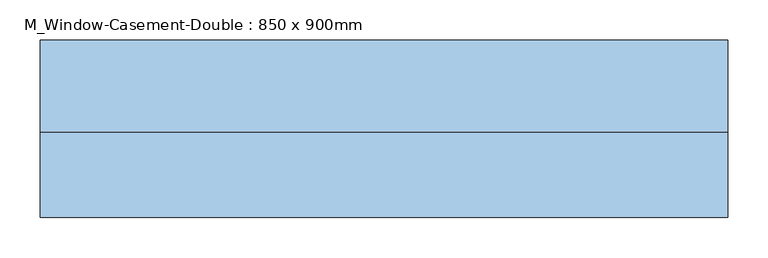
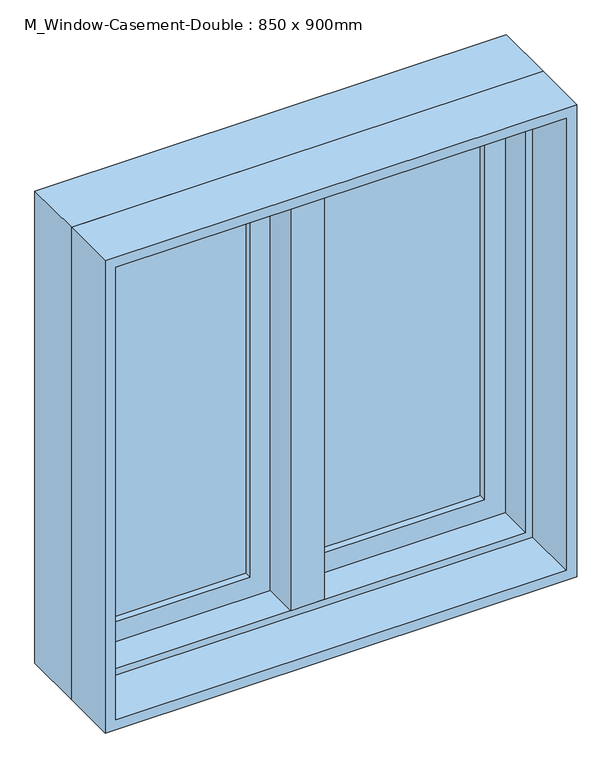
"""IFC4 building model written with IfcOpenShell, lengths in millimetres: window geometry, M_Window-Casement-Double : 850 x 900mm."""

from ifc_helpers import new_model, si_unit, frame, origin, place, context, project, spatial, polyline, outline, extrude, faceted_brep, source, transform, mapped, element, save


def m_window_casement_double_850_x_900mm_0f766704(model_context):
    return source(origin(), model_context, "Body", "SolidModel", [
        faceted_brep([(9.525, 119.05, 1787.3), (-9.525, 119.05, 1787.3), (-9.525, 68.25, 1787.3), (9.525, 68.25, 1787.3), (9.525, 119.05, 912.7), (9.525, 68.25, 912.7), (-9.525, 68.25, 912.7), (-9.525, 119.05, 912.7), (-9.525, 68.25, 931.75), (-9.525, 68.25, 1768.25), (-30.1625, 68.25, 931.75), (-30.1625, 68.25, 1768.25), (-30.1625, 4.75, 931.75), (-30.1625, 4.75, 1768.25), (30.1625, 4.75, 931.75), (30.1625, 4.75, 1768.25), (30.1625, 68.25, 931.75), (30.1625, 68.25, 1768.25), (9.525, 68.25, 931.75), (9.525, 68.25, 1768.25)], [[[0, 1, 2, 3]], [[4, 5, 6, 7]], [[1, 0, 4, 7]], [[2, 1, 7, 6, 8, 9]], [[9, 8, 10, 11]], [[11, 10, 12, 13]], [[13, 12, 14, 15]], [[15, 14, 16, 17]], [[17, 16, 18, 19]], [[0, 3, 19, 18, 5, 4]], [[18, 8, 6, 5]], [[9, 19, 3, 2]], [[8, 18, 16, 14, 12, 10]], [[19, 9, 11, 13, 15, 17]]]),
        extrude(outline(polyline([(-66.675, 100.0), (-66.675, 93.65), (-355.15, 93.65), (-355.15, 100.0), (-66.675, 100.0)])), frame((0.0, 0.0, 969.85), z_axis=(0.0, 0.0, 1.0), x_axis=(1.0, 0.0, 0.0)), (0.0, 0.0, 1.0), 760.3),
        extrude(outline(polyline([(-355.15, 80.95), (-355.15, 87.3), (-66.675, 87.3), (-66.675, 80.95), (-355.15, 80.95)])), frame((0.0, 0.0, 969.85), z_axis=(0.0, 0.0, 1.0), x_axis=(1.0, 0.0, 0.0)), (0.0, 0.0, 1.0), 760.3),
        extrude(outline(polyline([(355.15, 100.0), (355.15, 93.65), (66.675, 93.65), (66.675, 100.0), (355.15, 100.0)])), frame((0.0, 0.0, 969.85), z_axis=(0.0, 0.0, 1.0), x_axis=(1.0, 0.0, 0.0)), (0.0, 0.0, 1.0), 760.3),
        extrude(outline(polyline([(66.675, 80.95), (66.675, 87.3), (355.15, 87.3), (355.15, 80.95), (66.675, 80.95)])), frame((0.0, 0.0, 969.85), z_axis=(0.0, 0.0, 1.0), x_axis=(1.0, 0.0, 0.0)), (0.0, 0.0, 1.0), 760.3),
        extrude(outline(polyline([(1787.3, -412.3), (912.7, -412.3), (912.7, -9.525), (1787.3, -9.525), (1787.3, -412.3)]), holes=[polyline([(1730.15, -66.675), (969.85, -66.675), (969.85, -355.15), (1730.15, -355.15), (1730.15, -66.675)])]), frame((0.0, 68.25, 0.0), z_axis=(0.0, 1.0, 0.0), x_axis=(0.0, 0.0, 1.0)), (0.0, 0.0, 1.0), 44.45),
        extrude(outline(polyline([(912.7, 412.3), (1787.3, 412.3), (1787.3, 9.525), (912.7, 9.525), (912.7, 412.3)]), holes=[polyline([(969.85, 66.675), (1730.15, 66.675), (1730.15, 355.15), (969.85, 355.15), (969.85, 66.675)])]), frame((0.0, 68.25, 0.0), z_axis=(0.0, 1.0, 0.0), x_axis=(0.0, 0.0, 1.0)), (0.0, 0.0, 1.0), 44.45),
        extrude(outline(polyline([(1800.0, -425.0), (900.0, -425.0), (900.0, 425.0), (1800.0, 425.0), (1800.0, -425.0)]), holes=[polyline([(1780.95, 405.95), (919.05, 405.95), (919.05, -405.95), (1780.95, -405.95), (1780.95, 405.95)])]), frame((0.0, -100.0, 0.0), z_axis=(0.0, 1.0, 0.0), x_axis=(0.0, 0.0, 1.0)), (0.0, 0.0, 1.0), 104.75),
        faceted_brep([(393.25, 68.25, 1768.25), (393.25, 4.75, 1768.25), (-393.25, 4.75, 1768.25), (-393.25, 68.25, 1768.25), (412.3, 119.05, 1787.3), (412.3, 68.25, 1787.3), (-412.3, 68.25, 1787.3), (-412.3, 119.05, 1787.3), (425.0, 4.75, 1800.0), (425.0, 119.05, 1800.0), (-425.0, 119.05, 1800.0), (-425.0, 4.75, 1800.0), (-393.25, 4.75, 931.75), (-393.25, 68.25, 931.75), (-412.3, 68.25, 912.7), (-412.3, 119.05, 912.7), (-425.0, 119.05, 900.0), (-425.0, 4.75, 900.0), (393.25, 4.75, 931.75), (393.25, 68.25, 931.75), (412.3, 68.25, 912.7), (412.3, 119.05, 912.7), (425.0, 119.05, 900.0), (425.0, 4.75, 900.0)], [[[0, 1, 2, 3]], [[4, 5, 6, 7]], [[8, 9, 10, 11]], [[3, 2, 12, 13]], [[7, 6, 14, 15]], [[11, 10, 16, 17]], [[13, 12, 18, 19]], [[15, 14, 20, 21]], [[17, 16, 22, 23]], [[11, 17, 23, 8], [1, 18, 12, 2]], [[19, 18, 1, 0]], [[5, 20, 14, 6], [3, 13, 19, 0]], [[21, 20, 5, 4]], [[23, 22, 9, 8]], [[9, 22, 16, 10], [7, 15, 21, 4]]]),
    ])


if __name__ == "__main__":
    model = new_model("IFC4")
    model_context = context("Model", 3, world=origin())
    ifc_project = project(units=[si_unit("LENGTHUNIT", "METRE", prefix="MILLI")], contexts=[model_context])
    site = spatial("IfcSite", under=ifc_project)
    building = spatial("IfcBuilding", under=site)
    placement = place(None, origin())
    m_window_casement_double_850_x_900mm_shape = m_window_casement_double_850_x_900mm_0f766704(model_context)
    element("IfcWindow", 1, ObjectType="M_Window-Casement-Double : 850 x 900mm", at=placement, inside=building, context=model_context, shape_type="MappedRepresentation", body=[
        mapped(m_window_casement_double_850_x_900mm_shape, transform((0.0, 0.0, 0.0), x_axis=(1.0, 0.0, 0.0), y_axis=(0.0, 1.0, 0.0), z_axis=(0.0, 0.0, 1.0))),
    ])
    save(model, "model.ifc")

# Revit data of these elements
# Type "M_Window-Casement-Double : 850 x 900mm"
#   Type Mark = "23"
#   Fire Rating = "0.5h"
#   Assembly Code = "B2020100"
#   Analytic Construction = "Double glazing - domestic"
#   Frame Extension [instance default] = 0.020833 ft
#   Window Inset [instance default] = 0 ft
#   Wall Thickness [instance default] = 0.492126 ft
#   Interior Wall Closure [instance default] = 0.179626 ft
#   Half Width = 1.394357 ft
#   Visual Light Transmittance = 0.81
#   Thermal Resistance (R) = 0.319569 (m²·K)/W
#   Solar Heat Gain Coefficient = 0.76
#   Rough Width = 2.837927 ft
#   Rough Height = 3.001969 ft
#   Height = 2.952756 ft
#   Heat Transfer Coefficient (U) = 3.12929 W/(m²·K)
#   Exterior Wall Closure [instance default] = 0.104331 ft
#   Extension Jamb [instance default] = 0.179626 ft
#   Default Sill Height = 2.952756 ft
#   Width = 2.788714 ft
#   Define Thermal Properties by = 0
#   Muntin Visibility = yes
#   Interior Trim Visibility [instance default] = yes
#   Exterior Trim Visibility [instance default] = yes
#   Extension Jamb Visibility [instance default] = yes
#   Interior Trim Material = Wood - Stained
#   Muntin Pattern = M_Muntin Pattern_2x2 : M_Muntin Pattern_2x2
#   Interior Trim = M_Trim-Window-Interior-Flat : Picture Frame
#   Interior Frame Material = Wood - Stained
#   Glass Panel Material = Glass
#   Exterior Trim Material = Clad - White
#   Exterior Trim = M_Trim-Window-Exterior-Flat : with Sill
#   Exterior Frame Material = Clad - White
#   Wall Closure = (empty or 0)
# Element 1 (IfcWindow, "M_Window-Casement-Double : 850 x 900mm")
#   Wall Thickness = 0.656168 ft
#   Extension Jamb = 0.343668 ft
#   Materials on its faces: "Wood - Stained", "Glass", "Clad - White"
# Materials
#   "Wood - Stained": class "Wood", colour RGB 224 178 126, transparency 0, Cost = 0
#   "Glass": class "Glass", colour RGB 0 128 192, transparency 0.9, Description = "Soda Lime Glass", Cost = 0
#   "Clad - White": class "Wood", colour RGB 242 242 238, transparency 0, Cost = 0
